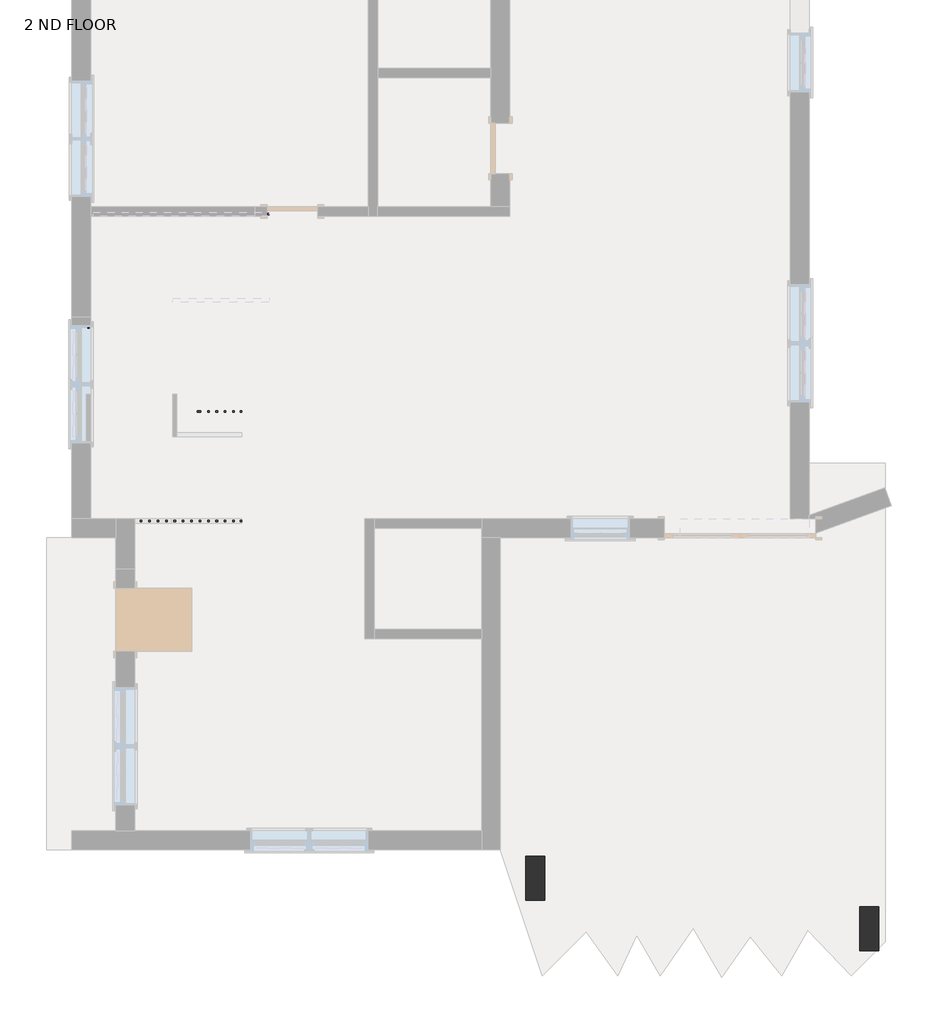
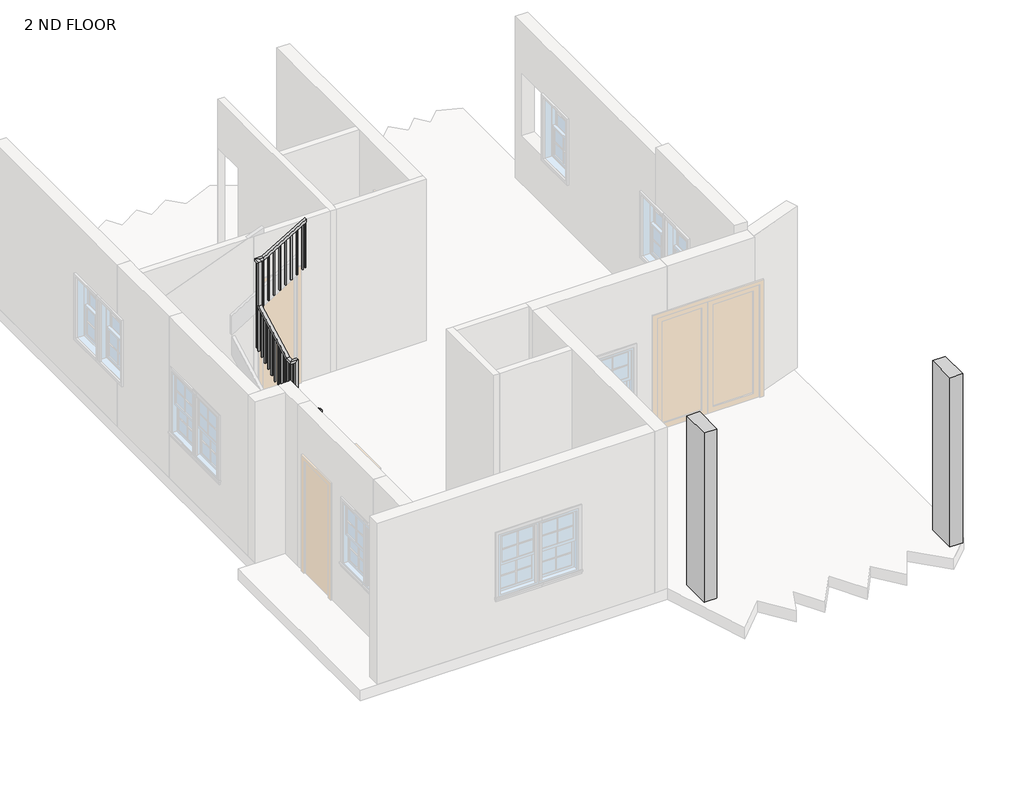
# One storey, part 2 of 3: 2 columns, 2 railings.
"""IFC4 building model written with IfcOpenShell, lengths in millimetres."""

from ifc_helpers import new_model, si_unit, frame, origin, place, context, project, spatial, polyline, outline, extrude, faceted_brep, transform, mapped, element, save
from components import column_8ec85f3f

model = new_model("IFC4")

# Units and contexts
model_context = context("Model", 3, world=origin())
ifc_project = project(units=[si_unit("LENGTHUNIT", "METRE", prefix="MILLI")], contexts=[model_context])

# Site, building, storey
site = spatial("IfcSite", under=ifc_project)
building = spatial("IfcBuilding", under=site)
storey = spatial("IfcBuildingStorey", under=building, Name="2 ND FLOOR", Elevation=6400.8)

# Columns
placement = place(None, origin())
column_shape = column_8ec85f3f(model_context)
element("IfcColumn", 1, ObjectType="Rectangular Column : x9\"", at=placement, inside=storey, context=model_context, shape_type="MappedRepresentation", body=[
    mapped(column_shape, transform((-16875.4750314, 319.9223646, 0.0), x_axis=(1.0, 0.0, 0.0), y_axis=(0.0, 1.0, 0.0), z_axis=(0.0, 0.0, 1.0))),
])
element("IfcColumn", 2, ObjectType="Rectangular Column : x9\"", at=placement, inside=storey, context=model_context, shape_type="MappedRepresentation", body=[
    mapped(column_shape, transform((-12836.8750314, -289.6776354, 0.0), x_axis=(1.0, 0.0, 0.0), y_axis=(0.0, 1.0, 0.0), z_axis=(0.0, 0.0, 1.0))),
])

# Railings
element("IfcRailing", 3, ObjectType="Handrail - Rectangular", at=placement, inside=storey, context=model_context, shape_type="SolidModel", body=[
    faceted_brep([(-20418.7750314, 5933.3223646, 7670.8), (-20418.7750314, 5933.3223646, 7610.586276), (-20418.7750314, 5984.1223646, 7610.586276), (-20418.7750314, 5984.1223646, 7670.8), (-20850.5750314, 5933.3223646, 7945.5818182), (-20901.3750314, 5933.3223646, 7917.6953669), (-20901.3750314, 5984.1223646, 7917.6953669), (-20850.5750314, 5984.1223646, 7945.5818182), (-20850.5750314, 5933.3223646, 8775.3151515), (-20901.3750314, 5933.3223646, 8724.5151515), (-20901.3750314, 5984.1223646, 8724.5151515), (-20850.5750314, 5984.1223646, 8775.3151515), (-20977.5750314, 5933.3223646, 8775.3151515), (-20977.5750314, 5933.3223646, 8724.5151515), (-20926.7750314, 5984.1223646, 8724.5151515), (-20926.7750314, 5984.1223646, 8775.3151515), (-20977.5750314, 6060.3223646, 8775.3151515), (-20977.5750314, 6072.9586335, 8724.5151515), (-20926.7750314, 6072.9586335, 8724.5151515), (-20926.7750314, 6060.3223646, 8775.3151515), (-20977.5750314, 6923.9223646, 9233.2848485), (-20977.5750314, 6974.7223646, 9202.7231907), (-20926.7750314, 6974.7223646, 9202.7231907), (-20926.7750314, 6923.9223646, 9233.2848485), (-20088.5750314, 7050.9223646, 10515.6), (-20088.5750314, 7000.1223646, 10515.6), (-20088.5750314, 7000.1223646, 10456.1290495), (-20088.5750314, 7050.9223646, 10456.1290495), (-20836.3298984, 7050.9223646, 10000.973913), (-20850.5750314, 7050.9223646, 10051.773913), (-20836.3298984, 7000.1223646, 10000.973913), (-20850.5750314, 7000.1223646, 10051.773913), (-20977.5750314, 6923.9223646, 10051.773913), (-20977.5750314, 6974.7223646, 10000.973913), (-20926.7750314, 6974.7223646, 10000.973913), (-20926.7750314, 6923.9223646, 10051.773913), (-20977.5750314, 7050.9223646, 10051.773913), (-20977.5750314, 7050.9223646, 10000.973913), (-20926.7750314, 7000.1223646, 10000.973913), (-20926.7750314, 7000.1223646, 10051.773913)], [[[0, 1, 2, 3]], [[1, 0, 4, 5]], [[2, 1, 5, 6]], [[3, 2, 6, 7]], [[0, 3, 7, 4]], [[5, 4, 8, 9]], [[6, 5, 9, 10]], [[7, 6, 10, 11]], [[4, 7, 11, 8]], [[9, 8, 12, 13]], [[10, 9, 13, 14]], [[11, 10, 14, 15]], [[8, 11, 15, 12]], [[13, 12, 16, 17]], [[14, 13, 17, 18]], [[15, 14, 18, 19]], [[12, 15, 19, 16]], [[17, 16, 20, 21]], [[18, 17, 21, 22]], [[19, 18, 22, 23]], [[16, 19, 23, 20]], [[24, 25, 26, 27]], [[28, 29, 24, 27]], [[30, 28, 27, 26]], [[31, 30, 26, 25]], [[29, 31, 25, 24]], [[21, 20, 32, 33]], [[22, 21, 33, 34]], [[23, 22, 34, 35]], [[20, 23, 35, 32]], [[33, 32, 36, 37]], [[34, 33, 37, 38]], [[35, 34, 38, 39]], [[32, 35, 39, 36]], [[37, 36, 29, 28]], [[38, 37, 28, 30]], [[39, 38, 30, 31]], [[36, 39, 31, 29]]]),
    extrude(outline(polyline([(10431.0051365, -20129.8500314), (10419.4094843, -20148.9000314), (9570.2782609, -20148.9000314), (9570.2782609, -20129.8500314), (10431.0051365, -20129.8500314)])), frame((0.0, 7015.9973646, 0.0), z_axis=(0.0, 1.0, 0.0), x_axis=(0.0, 0.0, 1.0)), (0.0, 0.0, 1.0), 19.05),
    extrude(outline(polyline([(10369.1616582, -20231.4500314), (10357.566006, -20250.5000314), (9508.4347826, -20250.5000314), (9508.4347826, -20231.4500314), (10369.1616582, -20231.4500314)])), frame((0.0, 7015.9973646, 0.0), z_axis=(0.0, 1.0, 0.0), x_axis=(0.0, 0.0, 1.0)), (0.0, 0.0, 1.0), 19.05),
    extrude(outline(polyline([(10307.31818, -20333.0500314), (10295.7225278, -20352.1000314), (9446.5913043, -20352.1000314), (9446.5913043, -20333.0500314), (10307.31818, -20333.0500314)])), frame((0.0, 7015.9973646, 0.0), z_axis=(0.0, 1.0, 0.0), x_axis=(0.0, 0.0, 1.0)), (0.0, 0.0, 1.0), 19.05),
    extrude(outline(polyline([(10245.4747017, -20434.6500314), (10233.8790495, -20453.7000314), (9384.7478261, -20453.7000314), (9384.7478261, -20434.6500314), (10245.4747017, -20434.6500314)])), frame((0.0, 7015.9973646, 0.0), z_axis=(0.0, 1.0, 0.0), x_axis=(0.0, 0.0, 1.0)), (0.0, 0.0, 1.0), 19.05),
    extrude(outline(polyline([(10183.6312234, -20536.2500314), (10172.0355713, -20555.3000314), (9322.9043478, -20555.3000314), (9322.9043478, -20536.2500314), (10183.6312234, -20536.2500314)])), frame((0.0, 7015.9973646, 0.0), z_axis=(0.0, 1.0, 0.0), x_axis=(0.0, 0.0, 1.0)), (0.0, 0.0, 1.0), 19.05),
    extrude(outline(polyline([(10121.7877452, -20637.8500314), (10110.192093, -20656.9000314), (9261.0608696, -20656.9000314), (9261.0608696, -20637.8500314), (10121.7877452, -20637.8500314)])), frame((0.0, 7015.9973646, 0.0), z_axis=(0.0, 1.0, 0.0), x_axis=(0.0, 0.0, 1.0)), (0.0, 0.0, 1.0), 19.05),
    extrude(outline(polyline([(10059.9442669, -20739.4500314), (10048.3486147, -20758.5000314), (9199.2173913, -20758.5000314), (9199.2173913, -20739.4500314), (10059.9442669, -20739.4500314)])), frame((0.0, 7015.9973646, 0.0), z_axis=(0.0, 1.0, 0.0), x_axis=(0.0, 0.0, 1.0)), (0.0, 0.0, 1.0), 19.05),
    extrude(outline(polyline([(9998.1007887, -20841.0500314), (9986.5051365, -20860.1000314), (9137.373913, -20860.1000314), (9137.373913, -20841.0500314), (9998.1007887, -20841.0500314)])), frame((0.0, 7015.9973646, 0.0), z_axis=(0.0, 1.0, 0.0), x_axis=(0.0, 0.0, 1.0)), (0.0, 0.0, 1.0), 19.05),
    extrude(outline(polyline([(-20942.6500314, 6965.1973646), (-20961.7000314, 6965.1973646), (-20961.7000314, 6984.2473646), (-20942.6500314, 6984.2473646), (-20942.6500314, 6965.1973646)])), frame((0.0, 0.0, 8345.8242424), z_axis=(0.0, 0.0, 1.0), x_axis=(1.0, 0.0, 0.0)), (0.0, 0.0, 1.0), 1655.1496706),
    extrude(outline(polyline([(6863.5973646, 9143.7932665), (6882.6473646, 9153.8955392), (6882.6473646, 8291.9454545), (6863.5973646, 8291.9454545), (6863.5973646, 9143.7932665)])), frame((-20961.7000314, 0.0, 0.0), z_axis=(1.0, 0.0, 0.0), x_axis=(0.0, 1.0, 0.0)), (0.0, 0.0, 1.0), 19.05),
    extrude(outline(polyline([(6761.9973646, 9089.9144786), (6781.0473646, 9100.0167513), (6781.0473646, 8238.0666667), (6761.9973646, 8238.0666667), (6761.9973646, 9089.9144786)])), frame((-20961.7000314, 0.0, 0.0), z_axis=(1.0, 0.0, 0.0), x_axis=(0.0, 1.0, 0.0)), (0.0, 0.0, 1.0), 19.05),
    extrude(outline(polyline([(6660.3973646, 9036.0356907), (6679.4473646, 9046.1379635), (6679.4473646, 8184.1878788), (6660.3973646, 8184.1878788), (6660.3973646, 9036.0356907)])), frame((-20961.7000314, 0.0, 0.0), z_axis=(1.0, 0.0, 0.0), x_axis=(0.0, 1.0, 0.0)), (0.0, 0.0, 1.0), 19.05),
    extrude(outline(polyline([(6558.7973646, 8982.1569029), (6577.8473646, 8992.2591756), (6577.8473646, 8130.3090909), (6558.7973646, 8130.3090909), (6558.7973646, 8982.1569029)])), frame((-20961.7000314, 0.0, 0.0), z_axis=(1.0, 0.0, 0.0), x_axis=(0.0, 1.0, 0.0)), (0.0, 0.0, 1.0), 19.05),
    extrude(outline(polyline([(6457.1973646, 8928.278115), (6476.2473646, 8938.3803877), (6476.2473646, 8076.430303), (6457.1973646, 8076.430303), (6457.1973646, 8928.278115)])), frame((-20961.7000314, 0.0, 0.0), z_axis=(1.0, 0.0, 0.0), x_axis=(0.0, 1.0, 0.0)), (0.0, 0.0, 1.0), 19.05),
    extrude(outline(polyline([(6355.5973646, 8874.3993271), (6374.6473646, 8884.5015998), (6374.6473646, 8022.5515152), (6355.5973646, 8022.5515152), (6355.5973646, 8874.3993271)])), frame((-20961.7000314, 0.0, 0.0), z_axis=(1.0, 0.0, 0.0), x_axis=(0.0, 1.0, 0.0)), (0.0, 0.0, 1.0), 19.05),
    extrude(outline(polyline([(6253.9973646, 8820.5205392), (6273.0473646, 8830.6228119), (6273.0473646, 7968.6727273), (6253.9973646, 7968.6727273), (6253.9973646, 8820.5205392)])), frame((-20961.7000314, 0.0, 0.0), z_axis=(1.0, 0.0, 0.0), x_axis=(0.0, 1.0, 0.0)), (0.0, 0.0, 1.0), 19.05),
    extrude(outline(polyline([(6152.3973646, 8766.6417513), (6171.4473646, 8776.7440241), (6171.4473646, 7914.7939394), (6152.3973646, 7914.7939394), (6152.3973646, 8766.6417513)])), frame((-20961.7000314, 0.0, 0.0), z_axis=(1.0, 0.0, 0.0), x_axis=(0.0, 1.0, 0.0)), (0.0, 0.0, 1.0), 19.05),
    extrude(outline(polyline([(6050.7973646, 8712.7629635), (6069.8473646, 8722.8652362), (6069.8473646, 7860.9151515), (6050.7973646, 7860.9151515), (6050.7973646, 8712.7629635)])), frame((-20961.7000314, 0.0, 0.0), z_axis=(1.0, 0.0, 0.0), x_axis=(0.0, 1.0, 0.0)), (0.0, 0.0, 1.0), 19.05),
    extrude(outline(polyline([(-20917.2500314, 5968.2473646), (-20917.2500314, 5949.1973646), (-20936.3000314, 5949.1973646), (-20936.3000314, 5968.2473646), (-20917.2500314, 5968.2473646)])), frame((0.0, 0.0, 7079.6727273), z_axis=(0.0, 0.0, 1.0), x_axis=(1.0, 0.0, 0.0)), (0.0, 0.0, 1.0), 1644.8424242),
    extrude(outline(polyline([(7863.1430941, -20815.6500314), (7875.2658214, -20834.7000314), (7015.0181818, -20834.7000314), (7015.0181818, -20815.6500314), (7863.1430941, -20815.6500314)])), frame((0.0, 5949.1973646, 0.0), z_axis=(0.0, 1.0, 0.0), x_axis=(0.0, 0.0, 1.0)), (0.0, 0.0, 1.0), 19.05),
    extrude(outline(polyline([(7798.4885487, -20714.0500314), (7810.611276, -20733.1000314), (6950.3636364, -20733.1000314), (6950.3636364, -20714.0500314), (7798.4885487, -20714.0500314)])), frame((0.0, 5949.1973646, 0.0), z_axis=(0.0, 1.0, 0.0), x_axis=(0.0, 0.0, 1.0)), (0.0, 0.0, 1.0), 19.05),
    extrude(outline(polyline([(7733.8340032, -20612.4500314), (7745.9567305, -20631.5000314), (6885.7090909, -20631.5000314), (6885.7090909, -20612.4500314), (7733.8340032, -20612.4500314)])), frame((0.0, 5949.1973646, 0.0), z_axis=(0.0, 1.0, 0.0), x_axis=(0.0, 0.0, 1.0)), (0.0, 0.0, 1.0), 19.05),
    extrude(outline(polyline([(7669.1794578, -20510.8500314), (7681.3021851, -20529.9000314), (6821.0545455, -20529.9000314), (6821.0545455, -20510.8500314), (7669.1794578, -20510.8500314)])), frame((0.0, 5949.1973646, 0.0), z_axis=(0.0, 1.0, 0.0), x_axis=(0.0, 0.0, 1.0)), (0.0, 0.0, 1.0), 19.05),
    extrude(outline(polyline([(-20942.6500314, 7015.9973646), (-20961.7000314, 7015.9973646), (-20961.7000314, 7035.0473646), (-20942.6500314, 7035.0473646), (-20942.6500314, 7015.9973646)])), frame((0.0, 0.0, 8372.7636364), z_axis=(0.0, 0.0, 1.0), x_axis=(1.0, 0.0, 0.0)), (0.0, 0.0, 1.0), 1628.2102767),
    extrude(outline(polyline([(-20942.6500314, 5968.2473646), (-20942.6500314, 5949.1973646), (-20961.7000314, 5949.1973646), (-20961.7000314, 5968.2473646), (-20942.6500314, 5968.2473646)])), frame((0.0, 0.0, 7095.8363636), z_axis=(0.0, 0.0, 1.0), x_axis=(1.0, 0.0, 0.0)), (0.0, 0.0, 1.0), 1628.6787879),
    extrude(outline(polyline([(10456.1290495, -20088.5750314), (10444.5333973, -20107.6250314), (9595.4021739, -20107.6250314), (9595.4021739, -20088.5750314), (10456.1290495, -20088.5750314)])), frame((0.0, 7015.9973646, 0.0), z_axis=(0.0, 1.0, 0.0), x_axis=(0.0, 0.0, 1.0)), (0.0, 0.0, 1.0), 19.05),
    extrude(outline(polyline([(7610.586276, -20418.7750314), (7622.7090032, -20437.8250314), (6762.4613636, -20437.8250314), (6762.4613636, -20418.7750314), (7610.586276, -20418.7750314)])), frame((0.0, 5949.1973646, 0.0), z_axis=(0.0, 1.0, 0.0), x_axis=(0.0, 0.0, 1.0)), (0.0, 0.0, 1.0), 19.05),
])
element("IfcRailing", 4, ObjectType="Handrail - Rectangular", at=placement, inside=storey, context=model_context, shape_type="SolidModel", body=[
    faceted_brep([(-20418.7750314, 4612.5223646, 7670.8), (-20418.7750314, 4612.5223646, 7616.2938354), (-20418.7750314, 4663.3223646, 7616.2938354), (-20418.7750314, 4663.3223646, 7670.8), (-22171.3752061, 4612.5223646, 8352.3667346), (-22222.1752061, 4612.5223646, 8317.6161256), (-22222.1752061, 4663.3223646, 8317.6161256), (-22171.3752061, 4663.3223646, 8352.3667346), (-22171.3752061, 4612.5223646, 8382.000068), (-22222.1752061, 4612.5223646, 8331.200068), (-22222.1752061, 4663.3223646, 8331.200068), (-22171.3752061, 4663.3223646, 8382.000068), (-22298.3752061, 4612.5223646, 8382.000068), (-22298.3752061, 4612.5223646, 8331.200068), (-22247.5752061, 4663.3223646, 8331.200068), (-22247.5752061, 4663.3223646, 8382.000068), (-22298.3752061, 4739.5223646, 8382.000068), (-22298.3752061, 4739.5223646, 8331.200068), (-22247.5752061, 4739.5223646, 8331.200068), (-22247.5752061, 4739.5223646, 8382.000068), (-22298.3752061, 8371.7223646, 8382.000068), (-22298.3752061, 8371.7223646, 8331.200068), (-22247.5752061, 8320.9223646, 8331.200068), (-22247.5752061, 8320.9223646, 8382.000068), (-20088.5750314, 8371.7223646, 8382.000068), (-20088.5750314, 8320.9223646, 8382.000068), (-20088.5750314, 8320.9223646, 8331.200068), (-20088.5750314, 8371.7223646, 8331.200068)], [[[0, 1, 2, 3]], [[1, 0, 4, 5]], [[2, 1, 5, 6]], [[3, 2, 6, 7]], [[0, 3, 7, 4]], [[5, 4, 8, 9]], [[6, 5, 9, 10]], [[7, 6, 10, 11]], [[4, 7, 11, 8]], [[9, 8, 12, 13]], [[10, 9, 13, 14]], [[11, 10, 14, 15]], [[8, 11, 15, 12]], [[13, 12, 16, 17]], [[14, 13, 17, 18]], [[15, 14, 18, 19]], [[12, 15, 19, 16]], [[17, 16, 20, 21]], [[18, 17, 21, 22]], [[19, 18, 22, 23]], [[16, 19, 23, 20]], [[24, 25, 26, 27]], [[21, 20, 24, 27]], [[22, 21, 27, 26]], [[23, 22, 26, 25]], [[20, 23, 25, 24]]]),
    extrude(outline(polyline([(-20148.9002061, 8355.8473646), (-20129.8502061, 8355.8473646), (-20129.8502061, 8336.7973646), (-20148.9002061, 8336.7973646), (-20148.9002061, 8355.8473646)])), frame((0.0, 0.0, 7467.600068), z_axis=(0.0, 0.0, 1.0), x_axis=(1.0, 0.0, 0.0)), (0.0, 0.0, 1.0), 863.6),
    extrude(outline(polyline([(-20250.5002061, 8355.8473646), (-20231.4502061, 8355.8473646), (-20231.4502061, 8336.7973646), (-20250.5002061, 8336.7973646), (-20250.5002061, 8355.8473646)])), frame((0.0, 0.0, 7467.600068), z_axis=(0.0, 0.0, 1.0), x_axis=(1.0, 0.0, 0.0)), (0.0, 0.0, 1.0), 863.6),
    extrude(outline(polyline([(-20352.1002061, 8355.8473646), (-20333.0502061, 8355.8473646), (-20333.0502061, 8336.7973646), (-20352.1002061, 8336.7973646), (-20352.1002061, 8355.8473646)])), frame((0.0, 0.0, 7467.600068), z_axis=(0.0, 0.0, 1.0), x_axis=(1.0, 0.0, 0.0)), (0.0, 0.0, 1.0), 863.6),
    extrude(outline(polyline([(-20453.7002061, 8355.8473646), (-20434.6502061, 8355.8473646), (-20434.6502061, 8336.7973646), (-20453.7002061, 8336.7973646), (-20453.7002061, 8355.8473646)])), frame((0.0, 0.0, 7467.600068), z_axis=(0.0, 0.0, 1.0), x_axis=(1.0, 0.0, 0.0)), (0.0, 0.0, 1.0), 863.6),
    extrude(outline(polyline([(-20555.3002061, 8355.8473646), (-20536.2502061, 8355.8473646), (-20536.2502061, 8336.7973646), (-20555.3002061, 8336.7973646), (-20555.3002061, 8355.8473646)])), frame((0.0, 0.0, 7467.600068), z_axis=(0.0, 0.0, 1.0), x_axis=(1.0, 0.0, 0.0)), (0.0, 0.0, 1.0), 863.6),
    extrude(outline(polyline([(-20656.9002061, 8355.8473646), (-20637.8502061, 8355.8473646), (-20637.8502061, 8336.7973646), (-20656.9002061, 8336.7973646), (-20656.9002061, 8355.8473646)])), frame((0.0, 0.0, 7467.600068), z_axis=(0.0, 0.0, 1.0), x_axis=(1.0, 0.0, 0.0)), (0.0, 0.0, 1.0), 863.6),
    extrude(outline(polyline([(-20758.5002061, 8355.8473646), (-20739.4502061, 8355.8473646), (-20739.4502061, 8336.7973646), (-20758.5002061, 8336.7973646), (-20758.5002061, 8355.8473646)])), frame((0.0, 0.0, 7467.600068), z_axis=(0.0, 0.0, 1.0), x_axis=(1.0, 0.0, 0.0)), (0.0, 0.0, 1.0), 863.6),
    extrude(outline(polyline([(-20860.1002061, 8355.8473646), (-20841.0502061, 8355.8473646), (-20841.0502061, 8336.7973646), (-20860.1002061, 8336.7973646), (-20860.1002061, 8355.8473646)])), frame((0.0, 0.0, 7467.600068), z_axis=(0.0, 0.0, 1.0), x_axis=(1.0, 0.0, 0.0)), (0.0, 0.0, 1.0), 863.6),
    extrude(outline(polyline([(-20961.7002061, 8355.8473646), (-20942.6502061, 8355.8473646), (-20942.6502061, 8336.7973646), (-20961.7002061, 8336.7973646), (-20961.7002061, 8355.8473646)])), frame((0.0, 0.0, 7467.600068), z_axis=(0.0, 0.0, 1.0), x_axis=(1.0, 0.0, 0.0)), (0.0, 0.0, 1.0), 863.6),
    extrude(outline(polyline([(-21063.3002061, 8355.8473646), (-21044.2502061, 8355.8473646), (-21044.2502061, 8336.7973646), (-21063.3002061, 8336.7973646), (-21063.3002061, 8355.8473646)])), frame((0.0, 0.0, 7467.600068), z_axis=(0.0, 0.0, 1.0), x_axis=(1.0, 0.0, 0.0)), (0.0, 0.0, 1.0), 863.6),
    extrude(outline(polyline([(-21164.9002061, 8355.8473646), (-21145.8502061, 8355.8473646), (-21145.8502061, 8336.7973646), (-21164.9002061, 8336.7973646), (-21164.9002061, 8355.8473646)])), frame((0.0, 0.0, 7467.600068), z_axis=(0.0, 0.0, 1.0), x_axis=(1.0, 0.0, 0.0)), (0.0, 0.0, 1.0), 863.6),
    extrude(outline(polyline([(-21266.5002061, 8355.8473646), (-21247.4502061, 8355.8473646), (-21247.4502061, 8336.7973646), (-21266.5002061, 8336.7973646), (-21266.5002061, 8355.8473646)])), frame((0.0, 0.0, 7467.600068), z_axis=(0.0, 0.0, 1.0), x_axis=(1.0, 0.0, 0.0)), (0.0, 0.0, 1.0), 863.6),
    extrude(outline(polyline([(-21368.1002061, 8355.8473646), (-21349.0502061, 8355.8473646), (-21349.0502061, 8336.7973646), (-21368.1002061, 8336.7973646), (-21368.1002061, 8355.8473646)])), frame((0.0, 0.0, 7467.600068), z_axis=(0.0, 0.0, 1.0), x_axis=(1.0, 0.0, 0.0)), (0.0, 0.0, 1.0), 863.6),
    extrude(outline(polyline([(-21469.7002061, 8355.8473646), (-21450.6502061, 8355.8473646), (-21450.6502061, 8336.7973646), (-21469.7002061, 8336.7973646), (-21469.7002061, 8355.8473646)])), frame((0.0, 0.0, 7467.600068), z_axis=(0.0, 0.0, 1.0), x_axis=(1.0, 0.0, 0.0)), (0.0, 0.0, 1.0), 863.6),
    extrude(outline(polyline([(-21571.3002061, 8355.8473646), (-21552.2502061, 8355.8473646), (-21552.2502061, 8336.7973646), (-21571.3002061, 8336.7973646), (-21571.3002061, 8355.8473646)])), frame((0.0, 0.0, 7467.600068), z_axis=(0.0, 0.0, 1.0), x_axis=(1.0, 0.0, 0.0)), (0.0, 0.0, 1.0), 863.6),
    extrude(outline(polyline([(-21672.9002061, 8355.8473646), (-21653.8502061, 8355.8473646), (-21653.8502061, 8336.7973646), (-21672.9002061, 8336.7973646), (-21672.9002061, 8355.8473646)])), frame((0.0, 0.0, 7467.600068), z_axis=(0.0, 0.0, 1.0), x_axis=(1.0, 0.0, 0.0)), (0.0, 0.0, 1.0), 863.6),
    extrude(outline(polyline([(-21774.5002061, 8355.8473646), (-21755.4502061, 8355.8473646), (-21755.4502061, 8336.7973646), (-21774.5002061, 8336.7973646), (-21774.5002061, 8355.8473646)])), frame((0.0, 0.0, 7467.600068), z_axis=(0.0, 0.0, 1.0), x_axis=(1.0, 0.0, 0.0)), (0.0, 0.0, 1.0), 863.6),
    extrude(outline(polyline([(-21876.1002061, 8355.8473646), (-21857.0502061, 8355.8473646), (-21857.0502061, 8336.7973646), (-21876.1002061, 8336.7973646), (-21876.1002061, 8355.8473646)])), frame((0.0, 0.0, 7467.600068), z_axis=(0.0, 0.0, 1.0), x_axis=(1.0, 0.0, 0.0)), (0.0, 0.0, 1.0), 863.6),
    extrude(outline(polyline([(-21977.7002061, 8355.8473646), (-21958.6502061, 8355.8473646), (-21958.6502061, 8336.7973646), (-21977.7002061, 8336.7973646), (-21977.7002061, 8355.8473646)])), frame((0.0, 0.0, 7467.600068), z_axis=(0.0, 0.0, 1.0), x_axis=(1.0, 0.0, 0.0)), (0.0, 0.0, 1.0), 863.6),
    extrude(outline(polyline([(-22079.3002061, 8355.8473646), (-22060.2502061, 8355.8473646), (-22060.2502061, 8336.7973646), (-22079.3002061, 8336.7973646), (-22079.3002061, 8355.8473646)])), frame((0.0, 0.0, 7467.600068), z_axis=(0.0, 0.0, 1.0), x_axis=(1.0, 0.0, 0.0)), (0.0, 0.0, 1.0), 863.6),
    extrude(outline(polyline([(-22180.9002061, 8355.8473646), (-22161.8502061, 8355.8473646), (-22161.8502061, 8336.7973646), (-22180.9002061, 8336.7973646), (-22180.9002061, 8355.8473646)])), frame((0.0, 0.0, 7467.600068), z_axis=(0.0, 0.0, 1.0), x_axis=(1.0, 0.0, 0.0)), (0.0, 0.0, 1.0), 863.6),
    extrude(outline(polyline([(-22282.5002061, 8285.9973646), (-22282.5002061, 8305.0473646), (-22263.4502061, 8305.0473646), (-22263.4502061, 8285.9973646), (-22282.5002061, 8285.9973646)])), frame((0.0, 0.0, 7467.600068), z_axis=(0.0, 0.0, 1.0), x_axis=(1.0, 0.0, 0.0)), (0.0, 0.0, 1.0), 863.6),
    extrude(outline(polyline([(-22282.5002061, 8184.3973646), (-22282.5002061, 8203.4473646), (-22263.4502061, 8203.4473646), (-22263.4502061, 8184.3973646), (-22282.5002061, 8184.3973646)])), frame((0.0, 0.0, 7467.600068), z_axis=(0.0, 0.0, 1.0), x_axis=(1.0, 0.0, 0.0)), (0.0, 0.0, 1.0), 863.6),
    extrude(outline(polyline([(-22282.5002061, 8082.7973646), (-22282.5002061, 8101.8473646), (-22263.4502061, 8101.8473646), (-22263.4502061, 8082.7973646), (-22282.5002061, 8082.7973646)])), frame((0.0, 0.0, 7467.600068), z_axis=(0.0, 0.0, 1.0), x_axis=(1.0, 0.0, 0.0)), (0.0, 0.0, 1.0), 863.6),
    extrude(outline(polyline([(-22282.5002061, 7981.1973646), (-22282.5002061, 8000.2473646), (-22263.4502061, 8000.2473646), (-22263.4502061, 7981.1973646), (-22282.5002061, 7981.1973646)])), frame((0.0, 0.0, 7467.600068), z_axis=(0.0, 0.0, 1.0), x_axis=(1.0, 0.0, 0.0)), (0.0, 0.0, 1.0), 863.6),
    extrude(outline(polyline([(-22282.5002061, 7879.5973646), (-22282.5002061, 7898.6473646), (-22263.4502061, 7898.6473646), (-22263.4502061, 7879.5973646), (-22282.5002061, 7879.5973646)])), frame((0.0, 0.0, 7467.600068), z_axis=(0.0, 0.0, 1.0), x_axis=(1.0, 0.0, 0.0)), (0.0, 0.0, 1.0), 863.6),
    extrude(outline(polyline([(-22282.5002061, 7777.9973646), (-22282.5002061, 7797.0473646), (-22263.4502061, 7797.0473646), (-22263.4502061, 7777.9973646), (-22282.5002061, 7777.9973646)])), frame((0.0, 0.0, 7467.600068), z_axis=(0.0, 0.0, 1.0), x_axis=(1.0, 0.0, 0.0)), (0.0, 0.0, 1.0), 863.6),
    extrude(outline(polyline([(-22282.5002061, 7676.3973646), (-22282.5002061, 7695.4473646), (-22263.4502061, 7695.4473646), (-22263.4502061, 7676.3973646), (-22282.5002061, 7676.3973646)])), frame((0.0, 0.0, 7467.600068), z_axis=(0.0, 0.0, 1.0), x_axis=(1.0, 0.0, 0.0)), (0.0, 0.0, 1.0), 863.6),
    extrude(outline(polyline([(-22282.5002061, 7574.7973646), (-22282.5002061, 7593.8473646), (-22263.4502061, 7593.8473646), (-22263.4502061, 7574.7973646), (-22282.5002061, 7574.7973646)])), frame((0.0, 0.0, 7467.600068), z_axis=(0.0, 0.0, 1.0), x_axis=(1.0, 0.0, 0.0)), (0.0, 0.0, 1.0), 863.6),
    extrude(outline(polyline([(-22282.5002061, 7473.1973646), (-22282.5002061, 7492.2473646), (-22263.4502061, 7492.2473646), (-22263.4502061, 7473.1973646), (-22282.5002061, 7473.1973646)])), frame((0.0, 0.0, 7467.600068), z_axis=(0.0, 0.0, 1.0), x_axis=(1.0, 0.0, 0.0)), (0.0, 0.0, 1.0), 863.6),
    extrude(outline(polyline([(-22282.5002061, 7371.5973646), (-22282.5002061, 7390.6473646), (-22263.4502061, 7390.6473646), (-22263.4502061, 7371.5973646), (-22282.5002061, 7371.5973646)])), frame((0.0, 0.0, 7467.600068), z_axis=(0.0, 0.0, 1.0), x_axis=(1.0, 0.0, 0.0)), (0.0, 0.0, 1.0), 863.6),
    extrude(outline(polyline([(-22282.5002061, 7269.9973646), (-22282.5002061, 7289.0473646), (-22263.4502061, 7289.0473646), (-22263.4502061, 7269.9973646), (-22282.5002061, 7269.9973646)])), frame((0.0, 0.0, 7467.600068), z_axis=(0.0, 0.0, 1.0), x_axis=(1.0, 0.0, 0.0)), (0.0, 0.0, 1.0), 863.6),
    extrude(outline(polyline([(-22282.5002061, 7168.3973646), (-22282.5002061, 7187.4473646), (-22263.4502061, 7187.4473646), (-22263.4502061, 7168.3973646), (-22282.5002061, 7168.3973646)])), frame((0.0, 0.0, 7467.600068), z_axis=(0.0, 0.0, 1.0), x_axis=(1.0, 0.0, 0.0)), (0.0, 0.0, 1.0), 863.6),
    extrude(outline(polyline([(-22282.5002061, 7066.7973646), (-22282.5002061, 7085.8473646), (-22263.4502061, 7085.8473646), (-22263.4502061, 7066.7973646), (-22282.5002061, 7066.7973646)])), frame((0.0, 0.0, 7467.600068), z_axis=(0.0, 0.0, 1.0), x_axis=(1.0, 0.0, 0.0)), (0.0, 0.0, 1.0), 863.6),
    extrude(outline(polyline([(-22282.5002061, 6965.1973646), (-22282.5002061, 6984.2473646), (-22263.4502061, 6984.2473646), (-22263.4502061, 6965.1973646), (-22282.5002061, 6965.1973646)])), frame((0.0, 0.0, 7467.600068), z_axis=(0.0, 0.0, 1.0), x_axis=(1.0, 0.0, 0.0)), (0.0, 0.0, 1.0), 863.6),
    extrude(outline(polyline([(6882.6473646, 8331.200068), (6882.6473646, 8324.6894652), (6863.5973646, 8314.5871925), (6863.5973646, 8331.200068), (6882.6473646, 8331.200068)])), frame((-22282.5002061, 0.0, 0.0), z_axis=(1.0, 0.0, 0.0), x_axis=(0.0, 1.0, 0.0)), (0.0, 0.0, 1.0), 19.05),
    extrude(outline(polyline([(6781.0473646, 8331.200068), (6781.0473646, 8270.8106774), (6761.9973646, 8260.7084046), (6761.9973646, 8331.200068), (6781.0473646, 8331.200068)])), frame((-22282.5002061, 0.0, 0.0), z_axis=(1.0, 0.0, 0.0), x_axis=(0.0, 1.0, 0.0)), (0.0, 0.0, 1.0), 19.05),
    extrude(outline(polyline([(6679.4473646, 8331.200068), (6679.4473646, 8216.9318895), (6660.3973646, 8206.8296168), (6660.3973646, 8331.200068), (6679.4473646, 8331.200068)])), frame((-22282.5002061, 0.0, 0.0), z_axis=(1.0, 0.0, 0.0), x_axis=(0.0, 1.0, 0.0)), (0.0, 0.0, 1.0), 19.05),
    extrude(outline(polyline([(6577.8473646, 8331.200068), (6577.8473646, 8163.0531016), (6558.7973646, 8152.9508289), (6558.7973646, 8331.200068), (6577.8473646, 8331.200068)])), frame((-22282.5002061, 0.0, 0.0), z_axis=(1.0, 0.0, 0.0), x_axis=(0.0, 1.0, 0.0)), (0.0, 0.0, 1.0), 19.05),
    extrude(outline(polyline([(6476.2473646, 8331.200068), (6476.2473646, 8109.1743137), (6457.1973646, 8099.072041), (6457.1973646, 8331.200068), (6476.2473646, 8331.200068)])), frame((-22282.5002061, 0.0, 0.0), z_axis=(1.0, 0.0, 0.0), x_axis=(0.0, 1.0, 0.0)), (0.0, 0.0, 1.0), 19.05),
    extrude(outline(polyline([(6374.6473646, 8331.200068), (6374.6473646, 8055.2955258), (6355.5973646, 8045.1932531), (6355.5973646, 8331.200068), (6374.6473646, 8331.200068)])), frame((-22282.5002061, 0.0, 0.0), z_axis=(1.0, 0.0, 0.0), x_axis=(0.0, 1.0, 0.0)), (0.0, 0.0, 1.0), 19.05),
    extrude(outline(polyline([(6273.0473646, 8331.200068), (6273.0473646, 8001.416738), (6253.9973646, 7991.3144652), (6253.9973646, 8331.200068), (6273.0473646, 8331.200068)])), frame((-22282.5002061, 0.0, 0.0), z_axis=(1.0, 0.0, 0.0), x_axis=(0.0, 1.0, 0.0)), (0.0, 0.0, 1.0), 19.05),
    extrude(outline(polyline([(6171.4473646, 8331.200068), (6171.4473646, 7947.5379501), (6152.3973646, 7937.4356774), (6152.3973646, 8331.200068), (6171.4473646, 8331.200068)])), frame((-22282.5002061, 0.0, 0.0), z_axis=(1.0, 0.0, 0.0), x_axis=(0.0, 1.0, 0.0)), (0.0, 0.0, 1.0), 19.05),
    extrude(outline(polyline([(6069.8473646, 8331.200068), (6069.8473646, 7893.6591622), (6050.7973646, 7883.5568895), (6050.7973646, 8331.200068), (6069.8473646, 8331.200068)])), frame((-22282.5002061, 0.0, 0.0), z_axis=(1.0, 0.0, 0.0), x_axis=(0.0, 1.0, 0.0)), (0.0, 0.0, 1.0), 19.05),
    extrude(outline(polyline([(5968.2473646, 8331.200068), (5968.2473646, 7839.7803743), (5949.1973646, 7829.6781016), (5949.1973646, 8331.200068), (5968.2473646, 8331.200068)])), frame((-22282.5002061, 0.0, 0.0), z_axis=(1.0, 0.0, 0.0), x_axis=(0.0, 1.0, 0.0)), (0.0, 0.0, 1.0), 19.05),
    extrude(outline(polyline([(5866.6473646, 8331.200068), (5866.6473646, 7785.9015865), (5847.5973646, 7775.7993137), (5847.5973646, 8331.200068), (5866.6473646, 8331.200068)])), frame((-22282.5002061, 0.0, 0.0), z_axis=(1.0, 0.0, 0.0), x_axis=(0.0, 1.0, 0.0)), (0.0, 0.0, 1.0), 19.05),
    extrude(outline(polyline([(5765.0473646, 8331.200068), (5765.0473646, 7732.0227986), (5745.9973646, 7721.9205258), (5745.9973646, 8331.200068), (5765.0473646, 8331.200068)])), frame((-22282.5002061, 0.0, 0.0), z_axis=(1.0, 0.0, 0.0), x_axis=(0.0, 1.0, 0.0)), (0.0, 0.0, 1.0), 19.05),
    extrude(outline(polyline([(5663.4473646, 8331.200068), (5663.4473646, 7678.1440107), (5644.3973646, 7668.041738), (5644.3973646, 8331.200068), (5663.4473646, 8331.200068)])), frame((-22282.5002061, 0.0, 0.0), z_axis=(1.0, 0.0, 0.0), x_axis=(0.0, 1.0, 0.0)), (0.0, 0.0, 1.0), 19.05),
    extrude(outline(polyline([(5561.8473646, 8331.200068), (5561.8473646, 7624.2652228), (5542.7973646, 7614.1629501), (5542.7973646, 8331.200068), (5561.8473646, 8331.200068)])), frame((-22282.5002061, 0.0, 0.0), z_axis=(1.0, 0.0, 0.0), x_axis=(0.0, 1.0, 0.0)), (0.0, 0.0, 1.0), 19.05),
    extrude(outline(polyline([(5460.2473646, 8331.200068), (5460.2473646, 7570.3864349), (5441.1973646, 7560.2841622), (5441.1973646, 8331.200068), (5460.2473646, 8331.200068)])), frame((-22282.5002061, 0.0, 0.0), z_axis=(1.0, 0.0, 0.0), x_axis=(0.0, 1.0, 0.0)), (0.0, 0.0, 1.0), 19.05),
    extrude(outline(polyline([(5358.6473646, 8331.200068), (5358.6473646, 7516.5076471), (5339.5973646, 7506.4053743), (5339.5973646, 8331.200068), (5358.6473646, 8331.200068)])), frame((-22282.5002061, 0.0, 0.0), z_axis=(1.0, 0.0, 0.0), x_axis=(0.0, 1.0, 0.0)), (0.0, 0.0, 1.0), 19.05),
    extrude(outline(polyline([(5257.0473646, 8331.200068), (5257.0473646, 7462.6288592), (5237.9973646, 7452.5265865), (5237.9973646, 8331.200068), (5257.0473646, 8331.200068)])), frame((-22282.5002061, 0.0, 0.0), z_axis=(1.0, 0.0, 0.0), x_axis=(0.0, 1.0, 0.0)), (0.0, 0.0, 1.0), 19.05),
    extrude(outline(polyline([(5155.4473646, 8331.200068), (5155.4473646, 7408.7500713), (5136.3973646, 7398.6477986), (5136.3973646, 8331.200068), (5155.4473646, 8331.200068)])), frame((-22282.5002061, 0.0, 0.0), z_axis=(1.0, 0.0, 0.0), x_axis=(0.0, 1.0, 0.0)), (0.0, 0.0, 1.0), 19.05),
    extrude(outline(polyline([(5053.8473646, 8331.200068), (5053.8473646, 7354.8712834), (5034.7973646, 7344.7690107), (5034.7973646, 8331.200068), (5053.8473646, 8331.200068)])), frame((-22282.5002061, 0.0, 0.0), z_axis=(1.0, 0.0, 0.0), x_axis=(0.0, 1.0, 0.0)), (0.0, 0.0, 1.0), 19.05),
    extrude(outline(polyline([(4952.2473646, 8331.200068), (4952.2473646, 7300.9924955), (4933.1973646, 7290.8902228), (4933.1973646, 8331.200068), (4952.2473646, 8331.200068)])), frame((-22282.5002061, 0.0, 0.0), z_axis=(1.0, 0.0, 0.0), x_axis=(0.0, 1.0, 0.0)), (0.0, 0.0, 1.0), 19.05),
    extrude(outline(polyline([(-22282.5002061, 4831.5973646), (-22282.5002061, 4850.6473646), (-22263.4502061, 4850.6473646), (-22263.4502061, 4831.5973646), (-22282.5002061, 4831.5973646)])), frame((0.0, 0.0, 7467.600068), z_axis=(0.0, 0.0, 1.0), x_axis=(1.0, 0.0, 0.0)), (0.0, 0.0, 1.0), 863.6),
    extrude(outline(polyline([(-22282.5002061, 4729.9973646), (-22282.5002061, 4749.0473646), (-22263.4502061, 4749.0473646), (-22263.4502061, 4729.9973646), (-22282.5002061, 4729.9973646)])), frame((0.0, 0.0, 7467.600068), z_axis=(0.0, 0.0, 1.0), x_axis=(1.0, 0.0, 0.0)), (0.0, 0.0, 1.0), 863.6),
    extrude(outline(polyline([(-22238.0500314, 4628.3973646), (-22257.1000314, 4628.3973646), (-22257.1000314, 4647.4473646), (-22238.0500314, 4647.4473646), (-22238.0500314, 4628.3973646)])), frame((0.0, 0.0, 7467.6), z_axis=(0.0, 0.0, 1.0), x_axis=(1.0, 0.0, 0.0)), (0.0, 0.0, 1.0), 863.600068),
    extrude(outline(polyline([(8291.686891, -22155.5000314), (7428.0888889, -22155.5000314), (7428.0888889, -22136.4500314), (8284.2785577, -22136.4500314), (8291.686891, -22155.5000314)])), frame((0.0, 4628.3973646, 0.0), z_axis=(0.0, 1.0, 0.0), x_axis=(0.0, 0.0, 1.0)), (0.0, 0.0, 1.0), 19.05),
    extrude(outline(polyline([(8252.1757799, -22053.9000314), (7388.5777778, -22053.9000314), (7388.5777778, -22034.8500314), (8244.7674465, -22034.8500314), (8252.1757799, -22053.9000314)])), frame((0.0, 4628.3973646, 0.0), z_axis=(0.0, 1.0, 0.0), x_axis=(0.0, 0.0, 1.0)), (0.0, 0.0, 1.0), 19.05),
    extrude(outline(polyline([(8212.6646688, -21952.3000314), (7349.0666667, -21952.3000314), (7349.0666667, -21933.2500314), (8205.2563354, -21933.2500314), (8212.6646688, -21952.3000314)])), frame((0.0, 4628.3973646, 0.0), z_axis=(0.0, 1.0, 0.0), x_axis=(0.0, 0.0, 1.0)), (0.0, 0.0, 1.0), 19.05),
    extrude(outline(polyline([(8173.1535577, -21850.7000314), (7147.7746925, -21850.7000314), (7147.7746925, -21831.6500314), (8165.7452243, -21831.6500314), (8173.1535577, -21850.7000314)])), frame((0.0, 4628.3973646, 0.0), z_axis=(0.0, 1.0, 0.0), x_axis=(0.0, 0.0, 1.0)), (0.0, 0.0, 1.0), 19.05),
    extrude(outline(polyline([(8133.6424465, -21749.1000314), (7147.7746925, -21749.1000314), (7147.7746925, -21730.0500314), (8126.2341132, -21730.0500314), (8133.6424465, -21749.1000314)])), frame((0.0, 4628.3973646, 0.0), z_axis=(0.0, 1.0, 0.0), x_axis=(0.0, 0.0, 1.0)), (0.0, 0.0, 1.0), 19.05),
    extrude(outline(polyline([(8094.1313354, -21647.5000314), (7147.7746925, -21647.5000314), (7147.7746925, -21628.4500314), (8086.7230021, -21628.4500314), (8094.1313354, -21647.5000314)])), frame((0.0, 4628.3973646, 0.0), z_axis=(0.0, 1.0, 0.0), x_axis=(0.0, 0.0, 1.0)), (0.0, 0.0, 1.0), 19.05),
    extrude(outline(polyline([(8054.6202243, -21545.9000314), (7147.7746925, -21545.9000314), (7147.7746925, -21526.8500314), (8047.211891, -21526.8500314), (8054.6202243, -21545.9000314)])), frame((0.0, 4628.3973646, 0.0), z_axis=(0.0, 1.0, 0.0), x_axis=(0.0, 0.0, 1.0)), (0.0, 0.0, 1.0), 19.05),
    extrude(outline(polyline([(8015.1091132, -21444.3000314), (7147.7746925, -21444.3000314), (7147.7746925, -21425.2500314), (8007.7007799, -21425.2500314), (8015.1091132, -21444.3000314)])), frame((0.0, 4628.3973646, 0.0), z_axis=(0.0, 1.0, 0.0), x_axis=(0.0, 0.0, 1.0)), (0.0, 0.0, 1.0), 19.05),
    extrude(outline(polyline([(7975.5980021, -21342.7000314), (7147.7746925, -21342.7000314), (7147.7746925, -21323.6500314), (7968.1896688, -21323.6500314), (7975.5980021, -21342.7000314)])), frame((0.0, 4628.3973646, 0.0), z_axis=(0.0, 1.0, 0.0), x_axis=(0.0, 0.0, 1.0)), (0.0, 0.0, 1.0), 19.05),
    extrude(outline(polyline([(7936.086891, -21241.1000314), (7136.7770181, -21241.1000314), (7130.2188214, -21222.0500314), (7928.6785577, -21222.0500314), (7936.086891, -21241.1000314)])), frame((0.0, 4628.3973646, 0.0), z_axis=(0.0, 1.0, 0.0), x_axis=(0.0, 0.0, 1.0)), (0.0, 0.0, 1.0), 19.05),
    extrude(outline(polyline([(7896.5757799, -21139.5000314), (7101.7999689, -21139.5000314), (7095.2417722, -21120.4500314), (7889.1674465, -21120.4500314), (7896.5757799, -21139.5000314)])), frame((0.0, 4628.3973646, 0.0), z_axis=(0.0, 1.0, 0.0), x_axis=(0.0, 0.0, 1.0)), (0.0, 0.0, 1.0), 19.05),
    extrude(outline(polyline([(7857.0646688, -21037.9000314), (7066.8229198, -21037.9000314), (7060.264723, -21018.8500314), (7849.6563354, -21018.8500314), (7857.0646688, -21037.9000314)])), frame((0.0, 4628.3973646, 0.0), z_axis=(0.0, 1.0, 0.0), x_axis=(0.0, 0.0, 1.0)), (0.0, 0.0, 1.0), 19.05),
    extrude(outline(polyline([(7817.5535577, -20936.3000314), (7031.8458706, -20936.3000314), (7025.2876739, -20917.2500314), (7810.1452243, -20917.2500314), (7817.5535577, -20936.3000314)])), frame((0.0, 4628.3973646, 0.0), z_axis=(0.0, 1.0, 0.0), x_axis=(0.0, 0.0, 1.0)), (0.0, 0.0, 1.0), 19.05),
    extrude(outline(polyline([(7778.0424465, -20834.7000314), (6996.8688214, -20834.7000314), (6990.3106247, -20815.6500314), (7770.6341132, -20815.6500314), (7778.0424465, -20834.7000314)])), frame((0.0, 4628.3973646, 0.0), z_axis=(0.0, 1.0, 0.0), x_axis=(0.0, 0.0, 1.0)), (0.0, 0.0, 1.0), 19.05),
    extrude(outline(polyline([(7738.5313354, -20733.1000314), (6961.8917722, -20733.1000314), (6955.3335755, -20714.0500314), (7731.1230021, -20714.0500314), (7738.5313354, -20733.1000314)])), frame((0.0, 4628.3973646, 0.0), z_axis=(0.0, 1.0, 0.0), x_axis=(0.0, 0.0, 1.0)), (0.0, 0.0, 1.0), 19.05),
    extrude(outline(polyline([(7699.0202243, -20631.5000314), (6926.914723, -20631.5000314), (6920.3565263, -20612.4500314), (7691.611891, -20612.4500314), (7699.0202243, -20631.5000314)])), frame((0.0, 4628.3973646, 0.0), z_axis=(0.0, 1.0, 0.0), x_axis=(0.0, 0.0, 1.0)), (0.0, 0.0, 1.0), 19.05),
    extrude(outline(polyline([(7659.5091132, -20529.9000314), (6891.9376739, -20529.9000314), (6885.3794771, -20510.8500314), (7652.1007799, -20510.8500314), (7659.5091132, -20529.9000314)])), frame((0.0, 4628.3973646, 0.0), z_axis=(0.0, 1.0, 0.0), x_axis=(0.0, 0.0, 1.0)), (0.0, 0.0, 1.0), 19.05),
    extrude(outline(polyline([(-22282.5002061, 8336.7973646), (-22282.5002061, 8355.8473646), (-22263.4502061, 8355.8473646), (-22263.4502061, 8336.7973646), (-22282.5002061, 8336.7973646)])), frame((0.0, 0.0, 7467.600068), z_axis=(0.0, 0.0, 1.0), x_axis=(1.0, 0.0, 0.0)), (0.0, 0.0, 1.0), 863.6),
    extrude(outline(polyline([(-22263.4502061, 4628.3973646), (-22282.5002061, 4628.3973646), (-22282.5002061, 4647.4473646), (-22263.4502061, 4647.4473646), (-22263.4502061, 4628.3973646)])), frame((0.0, 0.0, 7477.4778457), z_axis=(0.0, 0.0, 1.0), x_axis=(1.0, 0.0, 0.0)), (0.0, 0.0, 1.0), 853.7222222),
    extrude(outline(polyline([(-20107.6250314, 8355.8473646), (-20088.5750314, 8355.8473646), (-20088.5750314, 8336.7973646), (-20107.6250314, 8336.7973646), (-20107.6250314, 8355.8473646)])), frame((0.0, 0.0, 7467.600068), z_axis=(0.0, 0.0, 1.0), x_axis=(1.0, 0.0, 0.0)), (0.0, 0.0, 1.0), 863.6),
    extrude(outline(polyline([(7623.7021688, -20437.8250314), (6860.239723, -20437.8250314), (6853.6815263, -20418.7750314), (7616.2938354, -20418.7750314), (7623.7021688, -20437.8250314)])), frame((0.0, 4628.3973646, 0.0), z_axis=(0.0, 1.0, 0.0), x_axis=(0.0, 0.0, 1.0)), (0.0, 0.0, 1.0), 19.05),
])

save(model, "model.ifc")

# Revit data of these elements
# Type "Rectangular Column : x9\""
#   Assembly Code = "B1010200"
#   Depth = 1' - 9"
#   Offset Base = 0' - 0"
#   Offset Top = 0' - 0"
#   Width = 0' - 9"
#   Material = none
# Type "Handrail - Rectangular"
#   Assembly Code = "C2010400"
#   built-in parameter 1008612 = 0.0416667 (stored number, unit not read)
#   built-in parameter 1008611 = 0.0416667 (stored number, unit not read)
#   built-in parameter 1008609 = 0.333333 (stored number, unit not read)
#   built-in parameter 1008604 = 0.166667 (stored number, unit not read)
#   built-in parameter 1008603 = 0.166667 (stored number, unit not read)
#   Railing Height = 3' - 0"
#   built-in parameter 1008630 = 2
#   built-in parameter 1008610 = 2
#   built-in parameter 1008618 = Baluster - Square : 3/4"
# Elements 1, 2 (IfcColumn, "Rectangular Column : x9\"")
#   Phase Created = New Construction
# Elements 3, 4 (IfcRailing, "Handrail - Rectangular")
#   Phase Created = New Construction
